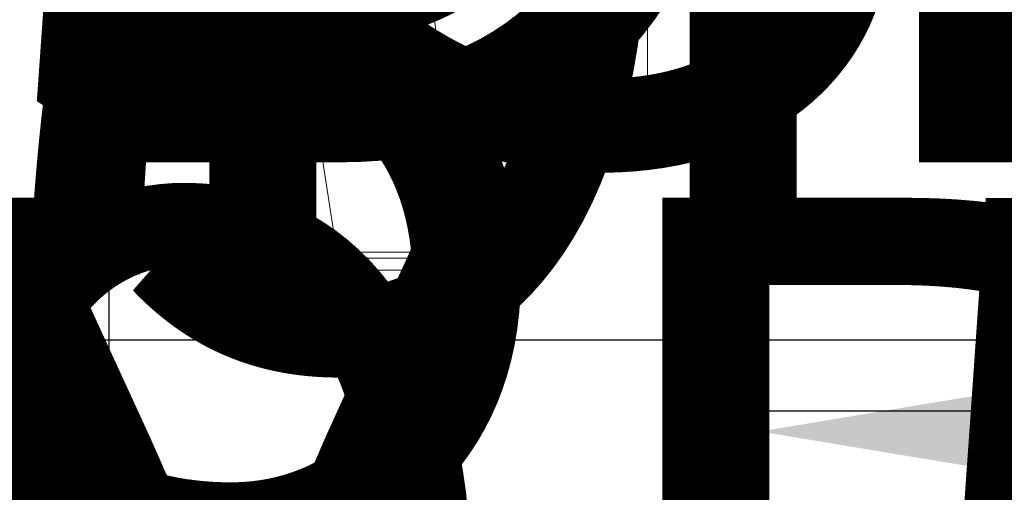
# Model space of a CAD drawing. Units: inches. Extents: x -307 to 2141, y -58 to 895.
# Tile 13 of 28: x 666 to 749, y 396 to 436. Entities that reach past the tile are written whole.
import ezdxf

# ---------------------------------------------------------------- set-up
doc = ezdxf.new("R2010")
doc.units = ezdxf.units.IN
doc.header["$MEASUREMENT"] = 0
doc.layers.add('A-ANNO-DIMS', color=2, linetype='Continuous', lineweight=18)
doc.layers.add('A-FURN', color=8, linetype='Continuous', lineweight=18)
doc.styles.get("Standard").update_dxf_attribs({"font": 'arial.ttf'})
doc.dimstyles.get("Standard").update_dxf_attribs({"dimtxt": 72, "dimasz": 48, "dimexe": 0.18, "dimexo": 0.0625, "dimgap": 0.09, "dimtad": 0, "dimtih": 1, "dimtoh": 1, "dimdec": 0, "dimrnd": 48, "dimzin": 0, "dimdsep": 46, "dimlunit": 3, "dimtxsty": 'Standard', "dimcen": 0.09, "dimadec": 0, "dimazin": 0, "dimtfac": 1, "dimtdec": 0, "dimtofl": 0, "dimtmove": 0, "dimatfit": 3, "dimfxl": 1, "dimtolj": 1, "dimtzin": 0, "dimarcsym": 0})

# ---------------------------------------------------------------- blocks, each defined once
blk = doc.blocks.new('Dining Set - 36 x 72 in.')
for p, q in [((36, 18), (-36, 18)), ((36, -18), (36, 18)), ((44.0006, 8.23428), (35.9976, 9.48474)), ((44, 8.23041), (44, -8.23915)), ((44.5, -8.15843), (44.5, 8.15338)), ((45.5, 8), (44.5005, 8.15617)), ((45.5, 8), (45.5, -8)), ((35.9976, -9.48476), (43.9993, -8.2345)), ((44.4997, -8.15631), (45.5, -8)), ((-36, -18), (36, -18))]:
    blk.add_line(p, q)
for points in [[(22.5879, 15.08984), (24.4721, 14.91715), (26.5052, 14.73958), (28.6809, 14.5581), (30.9929, 14.3737), (33.4347, 14.18733), (36, 14)], [(23.959, 11.37304), (25.2786, 11.08618), (26.8282, 10.76562), (28.6414, 10.40405), (30.752, 9.99414), (33.1936, 9.52856), (36, 9)], [(24.142, 6.64323), (24.4735, 6.70735), (24.8334, 6.75), (25.2235, 6.76969), (25.642, 6.76692), (26.0858, 6.74267), (26.5521, 6.69791), (27.0379, 6.63362), (27.5404, 6.55078), (28.0565, 6.45036), (28.5834, 6.33333), (29.1242, 6.19987), (29.7071, 6.04687), (30.3661, 5.87044), (31.1354, 5.66666), (32.0493, 5.43164), (33.142, 5.16146), (34.4475, 4.85221), (36, 4.5)], [(23.9549, -0.06836), (24.6146, 0.02083), (25.2235, 0.11784), (25.7904, 0.21875), (26.3241, 0.31966), (26.8334, 0.41666), (27.3265, 0.50618), (27.8099, 0.58593), (28.2894, 0.65397), (28.7709, 0.70833), (29.2601, 0.74707), (29.763, 0.76823), (30.2855, 0.76985), (30.8334, 0.75), (31.4088, 0.70784), (31.9994, 0.64713), (32.589, 0.57275), (33.1615, 0.48958), (33.7008, 0.4025), (34.1908, 0.3164), (34.6153, 0.23616), (34.9584, 0.16666), (35.2099, 0.11165), (35.3848, 0.07031), (35.504, 0.04069), (35.5886, 0.02083), (35.6594, 0.00879), (35.7377, 0.0026), (35.8442, 0.00032), (36, 0)], [(23.4727, -4.25391), (24.4289, -4.37549), (25.3334, -4.5), (26.1785, -4.62492), (26.9694, -4.74935), (27.7145, -4.87281), (28.4219, -4.99479), (29.1, -5.11483), (29.7572, -5.23242), (30.4016, -5.34709), (31.0417, -5.45834), (31.6837, -5.56437), (32.3262, -5.65821), (32.9658, -5.73153), (33.599, -5.77604), (34.2224, -5.78345), (34.8327, -5.74545), (35.4264, -5.65373), (36, -5.5)], [(23.9271, -8.76563), (24.9081, -8.82707), (25.8763, -8.89388), (26.8465, -8.96558), (27.8334, -9.04167), (28.8474, -9.12118), (29.8828, -9.20117), (30.93, -9.27824), (31.9792, -9.34896), (33.0205, -9.40991), (34.0443, -9.45768), (35.0407, -9.48885), (36, -9.5)], [(22.6615, -14.44271), (25.2312, -14.21509), (28.2624, -13.9069), (31.8277, -13.50594), (36, -13)]]:
    blk.add_lwpolyline(points)
blk = doc.blocks.new('*D26')
at = {"layer": 'A-ANNO-DIMS', "color": 0, "lineweight": -2, "transparency": 16777216}
for p, q in [((565.336, 584.202), (565.336, 572.085)), ((645.336, 584.202), (645.336, 572.085)), ((517.336, 572.265), (469.336, 572.265)), ((693.336, 572.265), (741.336, 572.265))]:
    blk.add_line(p, q, dxfattribs=at)
at = {"layer": 'A-ANNO-DIMS', "color": 0, "transparency": 16777216}
for points in [[(517.336, 580.265), (517.336, 564.265), (565.336, 572.265)], [(693.336, 580.265), (693.336, 564.265), (645.336, 572.265)]]:
    blk.add_solid(points, dxfattribs=at)
at = {"layer": 'Defpoints', "color": 0, "transparency": 16777216}
for p in [(565.336, 584.265), (645.336, 584.265), (565.336, 572.265)]:
    blk.add_point(p, dxfattribs=at)
at = {"layer": 'A-ANNO-DIMS', "color": 0, "transparency": 16777216, "insert": (178.225, 572.265), "char_height": 72, "attachment_point": 5}
blk.add_mtext('\\A1;BED 80 TYP.', dxfattribs=at)
blk = doc.blocks.new('*D28')
at = {"layer": 'A-ANNO-DIMS', "color": 0, "lineweight": -2, "transparency": 16777216}
for p, q in [((795.358, 433.55), (777.919, 433.55)), ((778.099, 385.55), (778.099, 366.073)), ((795.358, 318.073), (777.919, 318.073)), ((778.099, 318.073), (778.099, 270.073)), ((778.099, 270.073), (730.099, 270.073))]:
    blk.add_line(p, q, dxfattribs=at)
at = {"layer": 'A-ANNO-DIMS', "color": 0, "transparency": 16777216}
for points in [[(770.099, 385.55), (786.099, 385.55), (778.099, 433.55)], [(770.099, 366.073), (786.099, 366.073), (778.099, 318.073)]]:
    blk.add_solid(points, dxfattribs=at)
at = {"layer": 'Defpoints', "color": 0, "transparency": 16777216}
for p in [(795.421, 433.55), (778.099, 318.073), (795.421, 318.073)]:
    blk.add_point(p, dxfattribs=at)
at = {"layer": 'A-ANNO-DIMS', "color": 0, "transparency": 16777216, "insert": (534.416, 270.073), "char_height": 72, "attachment_point": 5}
blk.add_mtext('\\A1;BED 115', dxfattribs=at)
blk = doc.blocks.new('*D29')
at = {"layer": 'A-ANNO-DIMS', "color": 0, "lineweight": -2, "transparency": 16777216}
for p, q in [((747.421, 450.871), (699.421, 450.871)), ((795.421, 433.612), (795.421, 451.051)), ((882.028, 433.612), (882.028, 451.051)), ((930.028, 450.871), (978.028, 450.871))]:
    blk.add_line(p, q, dxfattribs=at)
at = {"layer": 'A-ANNO-DIMS', "color": 0, "transparency": 16777216}
for points in [[(747.421, 458.871), (747.421, 442.871), (795.421, 450.871)], [(930.028, 458.871), (930.028, 442.871), (882.028, 450.871)]]:
    blk.add_solid(points, dxfattribs=at)
at = {"layer": 'Defpoints', "color": 0, "transparency": 16777216}
for p in [(795.421, 450.871), (795.421, 433.55), (882.028, 433.55)]:
    blk.add_point(p, dxfattribs=at)
at = {"layer": 'A-ANNO-DIMS', "color": 0, "transparency": 16777216, "insert": (647.713, 450.871), "char_height": 72, "attachment_point": 5}
blk.add_mtext('\\A1;87', dxfattribs=at)
blk = doc.blocks.new('*D30')
at = {"layer": 'A-ANNO-DIMS', "color": 0, "lineweight": -2, "transparency": 16777216}
for p, q in [((570.736, 532.833), (570.736, 580.833)), ((570.736, 580.833), (618.736, 580.833)), ((565.398, 484.833), (570.916, 484.833)), ((565.398, 448.833), (570.916, 448.833)), ((570.736, 400.833), (570.736, 352.833))]:
    blk.add_line(p, q, dxfattribs=at)
at = {"layer": 'A-ANNO-DIMS', "color": 0, "transparency": 16777216}
for points in [[(562.736, 532.833), (578.736, 532.833), (570.736, 484.833)], [(562.736, 400.833), (578.736, 400.833), (570.736, 448.833)]]:
    blk.add_solid(points, dxfattribs=at)
at = {"layer": 'Defpoints', "color": 0, "transparency": 16777216}
for p in [(565.336, 484.833), (570.736, 484.833), (565.336, 448.833)]:
    blk.add_point(p, dxfattribs=at)
at = {"layer": 'A-ANNO-DIMS', "color": 0, "transparency": 16777216, "insert": (1030.174, 580.833), "char_height": 72, "attachment_point": 5}
blk.add_mtext('\\A1;WINDOW 36 TYP.', dxfattribs=at)
blk = doc.blocks.new('*D31')
at = {"layer": 'A-ANNO-DIMS', "color": 0, "lineweight": -2, "transparency": 16777216}
for p, q in [((556.336, 448.771), (556.336, 443.253)), ((565.336, 448.771), (565.336, 443.253)), ((508.336, 443.433), (460.336, 443.433)), ((613.336, 443.433), (661.336, 443.433))]:
    blk.add_line(p, q, dxfattribs=at)
at = {"layer": 'A-ANNO-DIMS', "color": 0, "transparency": 16777216}
for points in [[(508.336, 451.433), (508.336, 435.433), (556.336, 443.433)], [(613.336, 451.433), (613.336, 435.433), (565.336, 443.433)]]:
    blk.add_solid(points, dxfattribs=at)
at = {"layer": 'Defpoints', "color": 0, "transparency": 16777216}
for p in [(556.336, 448.833), (565.336, 448.833), (565.336, 443.433)]:
    blk.add_point(p, dxfattribs=at)
at = {"layer": 'A-ANNO-DIMS', "color": 0, "transparency": 16777216, "insert": (808.692, 443.433), "char_height": 72, "attachment_point": 5}
blk.add_mtext('\\A1;9 TYP.', dxfattribs=at)
blk = doc.blocks.new('*D35')
at = {"layer": 'A-ANNO-DIMS', "color": 0, "lineweight": -2, "transparency": 16777216}
for p, q in [((907.336, 443.029), (907.336, 453.949)), ((916.336, 443.029), (916.336, 453.949)), ((859.336, 453.769), (811.336, 453.769)), ((964.336, 453.769), (1012.336, 453.769))]:
    blk.add_line(p, q, dxfattribs=at)
at = {"layer": 'A-ANNO-DIMS', "color": 0, "transparency": 16777216}
for points in [[(859.336, 461.769), (859.336, 445.769), (907.336, 453.769)], [(964.336, 461.769), (964.336, 445.769), (916.336, 453.769)]]:
    blk.add_solid(points, dxfattribs=at)
at = {"layer": 'Defpoints', "color": 0, "transparency": 16777216}
for p in [(907.336, 453.769), (907.336, 442.967), (916.336, 442.967)]:
    blk.add_point(p, dxfattribs=at)
at = {"layer": 'A-ANNO-DIMS', "color": 0, "transparency": 16777216, "insert": (663.98, 453.769), "char_height": 72, "attachment_point": 5}
blk.add_mtext('\\A1;9 TYP.', dxfattribs=at)
blk = doc.blocks.new('*D36')
at = {"layer": 'A-ANNO-DIMS', "color": 0, "lineweight": -2, "transparency": 16777216}
for p, q in [((871.707, 562.404), (871.761, 610.404)), ((876.548, 514.399), (871.474, 514.405)), ((876.511, 481.353), (871.437, 481.358)), ((871.563, 433.358), (871.509, 385.358)), ((871.509, 385.358), (823.509, 385.358))]:
    blk.add_line(p, q, dxfattribs=at)
at = {"layer": 'A-ANNO-DIMS', "color": 0, "transparency": 16777216}
for points in [[(863.707, 562.413), (879.707, 562.395), (871.654, 514.404)], [(863.563, 433.367), (879.563, 433.349), (871.617, 481.358)]]:
    blk.add_solid(points, dxfattribs=at)
at = {"layer": 'Defpoints', "color": 0, "transparency": 16777216}
for p in [(876.611, 514.399), (871.617, 481.358), (876.574, 481.353)]:
    blk.add_point(p, dxfattribs=at)
at = {"layer": 'A-ANNO-DIMS', "color": 0, "transparency": 16777216, "insert": (548.95, 385.358), "char_height": 72, "attachment_point": 5}
blk.add_mtext('\\A1;WC 33 TYP.', dxfattribs=at)
blk = doc.blocks.new('*D37')
at = {"layer": 'A-ANNO-DIMS', "color": 0, "lineweight": -2, "transparency": 16777216}
for p, q in [((828.616, 519.409), (780.616, 519.463)), ((876.611, 514.461), (876.616, 519.536)), ((897.611, 514.438), (897.616, 519.512)), ((945.616, 519.279), (993.616, 519.225))]:
    blk.add_line(p, q, dxfattribs=at)
at = {"layer": 'A-ANNO-DIMS', "color": 0, "transparency": 16777216}
for points in [[(828.625, 527.409), (828.607, 511.409), (876.616, 519.356)], [(945.625, 527.279), (945.607, 511.279), (897.616, 519.332)]]:
    blk.add_solid(points, dxfattribs=at)
at = {"layer": 'Defpoints', "color": 0, "transparency": 16777216}
for p in [(876.616, 519.356), (876.611, 514.399), (897.611, 514.375)]:
    blk.add_point(p, dxfattribs=at)
at = {"layer": 'A-ANNO-DIMS', "color": 0, "transparency": 16777216, "insert": (604.676, 519.463), "char_height": 72, "attachment_point": 5}
blk.add_mtext('\\A1;21 TYP.', dxfattribs=at)
blk = doc.blocks.new('*D44')
at = {"layer": 'A-ANNO-DIMS', "color": 0, "lineweight": -2, "transparency": 16777216}
for p, q in [((815.327, 520.707), (815.406, 516.907)), ((839.872, 521.223), (839.952, 517.424)), ((887.938, 518.613), (935.927, 519.622)), ((767.413, 516.078), (719.424, 515.069))]:
    blk.add_line(p, q, dxfattribs=at)
at = {"layer": 'A-ANNO-DIMS', "color": 0, "transparency": 16777216}
for points in [[(887.769, 526.611), (888.106, 510.614), (839.948, 517.604)], [(767.245, 524.076), (767.581, 508.08), (815.403, 517.087)]]:
    blk.add_solid(points, dxfattribs=at)
at = {"layer": 'Defpoints', "color": 0, "transparency": 16777216}
for p in [(815.325, 520.769), (839.871, 521.285), (839.948, 517.604)]:
    blk.add_point(p, dxfattribs=at)
at = {"layer": 'A-ANNO-DIMS', "color": 0, "transparency": 16777216, "insert": (1151.157, 519.622), "char_height": 72, "attachment_point": 5}
blk.add_mtext('\\A1;BASIN 25', dxfattribs=at)
blk = doc.blocks.new('*D45')
at = {"layer": 'A-ANNO-DIMS', "color": 0, "lineweight": -2, "transparency": 16777216}
for p, q in [((841.111, 637.474), (793.111, 637.474)), ((842.12, 589.484), (841.111, 637.474)), ((839.51, 541.419), (843.309, 541.499)), ((839.933, 521.287), (843.732, 521.367)), ((844.562, 473.373), (845.571, 425.384))]:
    blk.add_line(p, q, dxfattribs=at)
at = {"layer": 'A-ANNO-DIMS', "color": 0, "transparency": 16777216}
for points in [[(850.118, 589.652), (834.122, 589.316), (843.129, 541.495)], [(852.56, 473.542), (836.563, 473.205), (843.553, 521.363)]]:
    blk.add_solid(points, dxfattribs=at)
at = {"layer": 'Defpoints', "color": 0, "transparency": 16777216}
for p in [(839.447, 541.417), (843.129, 541.495), (839.871, 521.285)]:
    blk.add_point(p, dxfattribs=at)
at = {"layer": 'A-ANNO-DIMS', "color": 0, "transparency": 16777216, "insert": (740.961, 637.474), "char_height": 72, "attachment_point": 5}
blk.add_mtext('\\A1;20', dxfattribs=at)
blk = doc.blocks.new('*D50')
at = {"layer": 'A-ANNO-DIMS', "color": 0, "lineweight": -2, "transparency": 16777216}
for p, q in [((565.336, 315.804), (565.336, 313.146)), ((582.271, 315.804), (582.271, 313.146)), ((517.336, 313.326), (469.336, 313.326)), ((630.271, 313.326), (678.271, 313.326))]:
    blk.add_line(p, q, dxfattribs=at)
at = {"layer": 'A-ANNO-DIMS', "color": 0, "transparency": 16777216}
for points in [[(517.336, 321.326), (517.336, 305.326), (565.336, 313.326)], [(630.271, 321.326), (630.271, 305.326), (582.271, 313.326)]]:
    blk.add_solid(points, dxfattribs=at)
at = {"layer": 'Defpoints', "color": 0, "transparency": 16777216}
for p in [(565.336, 315.867), (582.271, 315.867), (565.336, 313.326)]:
    blk.add_point(p, dxfattribs=at)
at = {"layer": 'A-ANNO-DIMS', "color": 0, "transparency": 16777216, "insert": (226.651, 313.326), "char_height": 72, "attachment_point": 5}
blk.add_mtext('\\A1;PHONE 17', dxfattribs=at)
blk = doc.blocks.new('*D51')
at = {"layer": 'A-ANNO-DIMS', "color": 0, "lineweight": -2, "transparency": 16777216}
for p, q in [((562.796, 379.109), (562.796, 427.109)), ((562.796, 427.109), (610.796, 427.109)), ((565.273, 331.109), (562.616, 331.109)), ((565.273, 315.867), (562.616, 315.867)), ((562.796, 267.867), (562.796, 219.867))]:
    blk.add_line(p, q, dxfattribs=at)
at = {"layer": 'A-ANNO-DIMS', "color": 0, "transparency": 16777216}
for points in [[(554.796, 379.109), (570.796, 379.109), (562.796, 331.109)], [(554.796, 267.867), (570.796, 267.867), (562.796, 315.867)]]:
    blk.add_solid(points, dxfattribs=at)
at = {"layer": 'Defpoints', "color": 0, "transparency": 16777216}
for p in [(562.796, 331.109), (565.336, 331.109), (565.336, 315.867)]:
    blk.add_point(p, dxfattribs=at)
at = {"layer": 'A-ANNO-DIMS', "color": 0, "transparency": 16777216, "insert": (659.336, 427.109), "char_height": 72, "attachment_point": 5}
blk.add_mtext('\\A1;15', dxfattribs=at)
blk = doc.blocks.new('*D52')
at = {"layer": 'A-ANNO-DIMS', "color": 0, "lineweight": -2, "transparency": 16777216}
for p, q in [((660.208, 554.249), (660.208, 602.249)), ((673.796, 506.249), (660.028, 506.249)), ((673.796, 415.249), (660.028, 415.249)), ((660.208, 367.249), (660.208, 319.249))]:
    blk.add_line(p, q, dxfattribs=at)
at = {"layer": 'A-ANNO-DIMS', "color": 0, "transparency": 16777216}
for points in [[(652.208, 554.249), (668.208, 554.249), (660.208, 506.249)], [(652.208, 367.249), (668.208, 367.249), (660.208, 415.249)]]:
    blk.add_solid(points, dxfattribs=at)
at = {"layer": 'Defpoints', "color": 0, "transparency": 16777216}
for p in [(673.858, 506.249), (660.208, 415.249), (673.858, 415.249)]:
    blk.add_point(p, dxfattribs=at)
at = {"layer": 'A-ANNO-DIMS', "color": 0, "transparency": 16777216, "insert": (660.208, 460.749), "char_height": 72, "attachment_point": 5}
blk.add_mtext('\\A1;DINING SET 91', dxfattribs=at)
blk = doc.blocks.new('*D53')
at = {"layer": 'A-ANNO-DIMS', "color": 0, "lineweight": -2, "transparency": 16777216}
for p, q in [((673.858, 415.186), (673.858, 401.419)), ((728.858, 415.186), (728.858, 401.419)), ((625.858, 401.599), (577.858, 401.599)), ((776.858, 401.599), (824.858, 401.599))]:
    blk.add_line(p, q, dxfattribs=at)
at = {"layer": 'A-ANNO-DIMS', "color": 0, "transparency": 16777216}
for points in [[(625.858, 409.599), (625.858, 393.599), (673.858, 401.599)], [(776.858, 409.599), (776.858, 393.599), (728.858, 401.599)]]:
    blk.add_solid(points, dxfattribs=at)
at = {"layer": 'Defpoints', "color": 0, "transparency": 16777216}
for p in [(673.858, 415.249), (728.858, 415.249), (728.858, 401.599)]:
    blk.add_point(p, dxfattribs=at)
at = {"layer": 'A-ANNO-DIMS', "color": 0, "transparency": 16777216, "insert": (876.787, 401.599), "char_height": 72, "attachment_point": 5}
blk.add_mtext('\\A1;55', dxfattribs=at)
blk = doc.blocks.new('*D54')
at = {"layer": 'A-ANNO-DIMS', "color": 0, "lineweight": -2, "transparency": 16777216}
for p, q in [((605.336, 412.349), (605.336, 460.349)), ((605.336, 460.349), (653.336, 460.349)), ((596.398, 364.349), (605.516, 364.349)), ((596.398, 304.349), (605.516, 304.349)), ((605.336, 256.349), (605.336, 208.349))]:
    blk.add_line(p, q, dxfattribs=at)
at = {"layer": 'A-ANNO-DIMS', "color": 0, "transparency": 16777216}
for points in [[(597.336, 412.349), (613.336, 412.349), (605.336, 364.349)], [(597.336, 256.349), (613.336, 256.349), (605.336, 304.349)]]:
    blk.add_solid(points, dxfattribs=at)
at = {"layer": 'Defpoints', "color": 0, "transparency": 16777216}
for p in [(596.336, 364.349), (605.336, 364.349), (596.336, 304.349)]:
    blk.add_point(p, dxfattribs=at)
at = {"layer": 'A-ANNO-DIMS', "color": 0, "transparency": 16777216, "insert": (854.004, 460.349), "char_height": 72, "attachment_point": 5}
blk.add_mtext('\\A1;DESK 60', dxfattribs=at)
blk = doc.blocks.new('*D55')
at = {"layer": 'A-ANNO-DIMS', "color": 0, "lineweight": -2, "transparency": 16777216}
for p, q in [((517.336, 373.349), (469.336, 373.349)), ((565.336, 364.411), (565.336, 373.529)), ((596.336, 364.411), (596.336, 373.529)), ((644.336, 373.349), (692.336, 373.349))]:
    blk.add_line(p, q, dxfattribs=at)
at = {"layer": 'A-ANNO-DIMS', "color": 0, "transparency": 16777216}
for points in [[(517.336, 381.349), (517.336, 365.349), (565.336, 373.349)], [(644.336, 381.349), (644.336, 365.349), (596.336, 373.349)]]:
    blk.add_solid(points, dxfattribs=at)
at = {"layer": 'Defpoints', "color": 0, "transparency": 16777216}
for p in [(565.336, 373.349), (565.336, 364.349), (596.336, 364.349)]:
    blk.add_point(p, dxfattribs=at)
at = {"layer": 'A-ANNO-DIMS', "color": 0, "transparency": 16777216, "insert": (424.651, 373.349), "char_height": 72, "attachment_point": 5}
blk.add_mtext('\\A1;31', dxfattribs=at)
blk = doc.blocks.new('*D60')
at = {"layer": 'A-ANNO-DIMS', "color": 0, "lineweight": -2, "transparency": 16777216}
for p, q in [((659.857, 294.946), (659.857, 342.946)), ((659.857, 342.946), (707.857, 342.946)), ((663.339, 246.946), (659.677, 246.946)), ((663.339, 223.315), (659.677, 223.315)), ((659.857, 175.315), (659.857, 127.315))]:
    blk.add_line(p, q, dxfattribs=at)
at = {"layer": 'A-ANNO-DIMS', "color": 0, "transparency": 16777216}
for points in [[(651.857, 294.946), (667.857, 294.946), (659.857, 246.946)], [(651.857, 175.315), (667.857, 175.315), (659.857, 223.315)]]:
    blk.add_solid(points, dxfattribs=at)
at = {"layer": 'Defpoints', "color": 0, "transparency": 16777216}
for p in [(659.857, 246.946), (663.402, 246.946), (663.402, 223.315)]:
    blk.add_point(p, dxfattribs=at)
at = {"layer": 'A-ANNO-DIMS', "color": 0, "transparency": 16777216, "insert": (933.573, 342.946), "char_height": 72, "attachment_point": 5}
blk.add_mtext('\\A1;TABLE 24', dxfattribs=at)
blk = doc.blocks.new('*D63')
at = {"layer": 'A-ANNO-DIMS', "color": 0, "lineweight": -2, "transparency": 16777216}
for p, q in [((916.398, 691.341), (947.72, 691.341)), ((947.54, 643.341), (947.54, 416.192)), ((947.54, 115.341), (947.54, 342.49)), ((704.684, 67.341), (947.72, 67.341))]:
    blk.add_line(p, q, dxfattribs=at)
at = {"layer": 'A-ANNO-DIMS', "color": 0, "transparency": 16777216}
for points in [[(939.54, 643.341), (955.54, 643.341), (947.54, 691.341)], [(939.54, 115.341), (955.54, 115.341), (947.54, 67.341)]]:
    blk.add_solid(points, dxfattribs=at)
at = {"layer": 'Defpoints', "color": 0, "transparency": 16777216}
for p in [(916.336, 691.341), (704.621, 67.341), (947.54, 67.341)]:
    blk.add_point(p, dxfattribs=at)
at = {"layer": 'A-ANNO-DIMS', "color": 0, "transparency": 16777216, "insert": (947.54, 379.341), "char_height": 72, "attachment_point": 5}
blk.add_mtext('\\A1;624', dxfattribs=at)
blk = doc.blocks.new('*D68')
at = {"layer": 'A-ANNO-DIMS', "color": 0, "lineweight": -2, "transparency": 16777216}
for p, q in [((525.132, 586.341), (525.132, 634.341)), ((525.132, 634.341), (573.132, 634.341)), ((565.273, 538.341), (524.952, 538.341)), ((556.273, 484.833), (524.952, 484.833)), ((525.132, 436.833), (525.132, 388.833))]:
    blk.add_line(p, q, dxfattribs=at)
at = {"layer": 'A-ANNO-DIMS', "color": 0, "transparency": 16777216}
for points in [[(517.132, 586.341), (533.132, 586.341), (525.132, 538.341)], [(517.132, 436.833), (533.132, 436.833), (525.132, 484.833)]]:
    blk.add_solid(points, dxfattribs=at)
at = {"layer": 'Defpoints', "color": 0, "transparency": 16777216}
for p in [(525.132, 538.341), (565.336, 538.341), (556.336, 484.833)]:
    blk.add_point(p, dxfattribs=at)
at = {"layer": 'A-ANNO-DIMS', "color": 0, "transparency": 16777216, "insert": (687.754, 634.341), "char_height": 72, "attachment_point": 5}
blk.add_mtext('\\A1;53.51', dxfattribs=at)
blk = doc.blocks.new('*D82')
at = {"layer": 'A-ANNO-DIMS', "color": 0, "lineweight": -2, "transparency": 16777216}
for p, q in [((525.132, 565.341), (525.132, 613.341)), ((525.132, 613.341), (573.132, 613.341)), ((802.273, 517.341), (524.952, 517.341)), ((802.273, 481.341), (524.952, 481.341)), ((525.132, 433.341), (525.132, 385.341))]:
    blk.add_line(p, q, dxfattribs=at)
at = {"layer": 'A-ANNO-DIMS', "color": 0, "transparency": 16777216}
for points in [[(517.132, 565.341), (533.132, 565.341), (525.132, 517.341)], [(517.132, 433.341), (533.132, 433.341), (525.132, 481.341)]]:
    blk.add_solid(points, dxfattribs=at)
at = {"layer": 'Defpoints', "color": 0, "transparency": 16777216}
for p in [(525.132, 517.341), (802.336, 517.341), (802.336, 481.341)]:
    blk.add_point(p, dxfattribs=at)
at = {"layer": 'A-ANNO-DIMS', "color": 0, "transparency": 16777216, "insert": (624.742, 613.341), "char_height": 72, "attachment_point": 5}
blk.add_mtext('\\A1;36', dxfattribs=at)
blk = doc.blocks.new('*D83')
at = {"layer": 'A-ANNO-DIMS', "color": 0, "lineweight": -2, "transparency": 16777216}
for p, q in [((947.54, 538.903), (947.54, 586.903)), ((916.398, 490.903), (947.72, 490.903)), ((907.398, 481.341), (947.72, 481.341)), ((947.54, 433.341), (947.54, 385.341)), ((947.54, 385.341), (899.54, 385.341))]:
    blk.add_line(p, q, dxfattribs=at)
at = {"layer": 'A-ANNO-DIMS', "color": 0, "transparency": 16777216}
for points in [[(939.54, 538.903), (955.54, 538.903), (947.54, 490.903)], [(939.54, 433.341), (955.54, 433.341), (947.54, 481.341)]]:
    blk.add_solid(points, dxfattribs=at)
at = {"layer": 'Defpoints', "color": 0, "transparency": 16777216}
for p in [(916.336, 490.903), (907.336, 481.341), (947.54, 481.341)]:
    blk.add_point(p, dxfattribs=at)
at = {"layer": 'A-ANNO-DIMS', "color": 0, "transparency": 16777216, "insert": (777.968, 385.341), "char_height": 72, "attachment_point": 5}
blk.add_mtext('\\A1;9.563', dxfattribs=at)
blk = doc.blocks.new('*D88')
at = {"layer": 'A-ANNO-DIMS', "color": 0, "lineweight": -2, "transparency": 16777216}
for p, q in [((517.33584, 722.544828), (469.33584, 722.544828)), ((565.33584, 295.403328), (565.33584, 722.724828)), ((754.33584, 271.403328), (754.33584, 722.724828)), ((802.33584, 722.544828), (850.33584, 722.544828))]:
    blk.add_line(p, q, dxfattribs=at)
at = {"layer": 'A-ANNO-DIMS', "color": 0, "transparency": 16777216}
for points in [[(517.33584, 730.544828), (517.33584, 714.544828), (565.33584, 722.544828)], [(802.33584, 730.544828), (802.33584, 714.544828), (754.33584, 722.544828)]]:
    blk.add_solid(points, dxfattribs=at)
at = {"layer": 'Defpoints', "color": 0, "transparency": 16777216}
for p in [(754.33584, 722.544828), (565.33584, 295.340828), (754.33584, 271.340828)]:
    blk.add_point(p, dxfattribs=at)
at = {"layer": 'A-ANNO-DIMS', "color": 0, "transparency": 16777216, "insert": (659.83584, 722.544828), "char_height": 72, "attachment_point": 5}
blk.add_mtext('\\A1;189', dxfattribs=at)
blk = doc.blocks.new('*D95')
at = {"layer": 'A-ANNO-DIMS', "color": 0, "lineweight": -2, "transparency": 16777216}
for p, q in [((947.54, 577.341), (947.54, 625.341)), ((947.54, 625.341), (995.54, 625.341)), ((629.898, 529.341), (947.72, 529.341)), ((629.898, 502.663), (947.72, 502.663)), ((947.54, 454.663), (947.54, 406.663))]:
    blk.add_line(p, q, dxfattribs=at)
at = {"layer": 'A-ANNO-DIMS', "color": 0, "transparency": 16777216}
for points in [[(939.54, 577.341), (955.54, 577.341), (947.54, 529.341)], [(939.54, 454.663), (955.54, 454.663), (947.54, 502.663)]]:
    blk.add_solid(points, dxfattribs=at)
at = {"layer": 'Defpoints', "color": 0, "transparency": 16777216}
for p in [(629.836, 529.341), (947.54, 529.341), (629.836, 502.663)]:
    blk.add_point(p, dxfattribs=at)
at = {"layer": 'A-ANNO-DIMS', "color": 0, "transparency": 16777216, "insert": (1117.799, 625.341), "char_height": 72, "attachment_point": 5}
blk.add_mtext('\\A1;26.68', dxfattribs=at)
blk = doc.blocks.new('*D99')
at = {"layer": 'A-ANNO-DIMS', "color": 0, "lineweight": -2, "transparency": 16777216}
for p, q in [((763.336, 481.278), (763.336, 35.957)), ((802.336, 481.278), (802.336, 35.957)), ((715.336, 36.137), (667.336, 36.137)), ((850.336, 36.137), (898.336, 36.137))]:
    blk.add_line(p, q, dxfattribs=at)
at = {"layer": 'A-ANNO-DIMS', "color": 0, "transparency": 16777216}
for points in [[(715.336, 44.137), (715.336, 28.137), (763.336, 36.137)], [(850.336, 44.137), (850.336, 28.137), (802.336, 36.137)]]:
    blk.add_solid(points, dxfattribs=at)
at = {"layer": 'Defpoints', "color": 0, "transparency": 16777216}
for p in [(763.336, 481.341), (802.336, 481.341), (802.336, 36.137)]:
    blk.add_point(p, dxfattribs=at)
at = {"layer": 'A-ANNO-DIMS', "color": 0, "transparency": 16777216, "insert": (950.044, 36.137), "char_height": 72, "attachment_point": 5}
blk.add_mtext('\\A1;39', dxfattribs=at)
blk = doc.blocks.new('*D100')
at = {"layer": 'A-ANNO-DIMS', "color": 0, "lineweight": -2, "transparency": 16777216}
for p, q in [((589.339, 409.278), (589.339, 35.957)), ((625.336, 409.278), (625.336, 35.957)), ((541.339, 36.137), (493.339, 36.137)), ((673.336, 36.137), (721.336, 36.137))]:
    blk.add_line(p, q, dxfattribs=at)
at = {"layer": 'A-ANNO-DIMS', "color": 0, "transparency": 16777216}
for points in [[(541.339, 44.137), (541.339, 28.137), (589.339, 36.137)], [(673.336, 44.137), (673.336, 28.137), (625.336, 36.137)]]:
    blk.add_solid(points, dxfattribs=at)
at = {"layer": 'Defpoints', "color": 0, "transparency": 16777216}
for p in [(589.339, 409.341), (625.336, 409.341), (625.336, 36.137)]:
    blk.add_point(p, dxfattribs=at)
at = {"layer": 'A-ANNO-DIMS', "color": 0, "transparency": 16777216, "insert": (772.946, 36.137), "char_height": 72, "attachment_point": 5}
blk.add_mtext('\\A1;36', dxfattribs=at)
blk = doc.blocks.new('*D107')
at = {"layer": 'A-ANNO-DIMS', "color": 0, "lineweight": -2, "transparency": 16777216}
for p, q in [((517.336, 722.545), (469.336, 722.545)), ((565.336, 409.403), (565.336, 722.725)), ((589.339, 409.403), (589.339, 722.725)), ((637.339, 722.545), (685.339, 722.545))]:
    blk.add_line(p, q, dxfattribs=at)
at = {"layer": 'A-ANNO-DIMS', "color": 0, "transparency": 16777216}
for points in [[(517.336, 730.545), (517.336, 714.545), (565.336, 722.545)], [(637.339, 730.545), (637.339, 714.545), (589.339, 722.545)]]:
    blk.add_solid(points, dxfattribs=at)
at = {"layer": 'Defpoints', "color": 0, "transparency": 16777216}
for p in [(589.339, 722.545), (565.336, 409.341), (589.339, 409.341)]:
    blk.add_point(p, dxfattribs=at)
at = {"layer": 'A-ANNO-DIMS', "color": 0, "transparency": 16777216, "insert": (835.495, 722.545), "char_height": 72, "attachment_point": 5}
blk.add_mtext('\\A1;24.003', dxfattribs=at)
blk = doc.blocks.new('*D108')
at = {"layer": 'A-ANNO-DIMS', "color": 0, "lineweight": -2, "transparency": 16777216}
for p, q in [((947.54, 550.663), (947.54, 598.663)), ((589.402, 502.663), (947.72, 502.663)), ((589.402, 409.341), (947.72, 409.341)), ((947.54, 361.341), (947.54, 313.341))]:
    blk.add_line(p, q, dxfattribs=at)
at = {"layer": 'A-ANNO-DIMS', "color": 0, "transparency": 16777216}
for points in [[(939.54, 550.663), (955.54, 550.663), (947.54, 502.663)], [(939.54, 361.341), (955.54, 361.341), (947.54, 409.341)]]:
    blk.add_solid(points, dxfattribs=at)
at = {"layer": 'Defpoints', "color": 0, "transparency": 16777216}
for p in [(589.339, 502.663), (947.54, 502.663), (589.339, 409.341)]:
    blk.add_point(p, dxfattribs=at)
at = {"layer": 'A-ANNO-DIMS', "color": 0, "transparency": 16777216, "insert": (947.54, 456.002), "char_height": 72, "attachment_point": 5}
blk.add_mtext('\\A1;93.32', dxfattribs=at)
blk = doc.blocks.new('*D109')
at = {"layer": 'A-ANNO-DIMS', "color": 0, "lineweight": -2, "transparency": 16777216}
for p, q in [((723.132, 355.341), (723.132, 403.341)), ((723.132, 403.341), (771.132, 403.341)), ((754.273, 307.341), (722.952, 307.341)), ((754.273, 271.341), (722.952, 271.341)), ((723.132, 223.341), (723.132, 175.341))]:
    blk.add_line(p, q, dxfattribs=at)
at = {"layer": 'A-ANNO-DIMS', "color": 0, "transparency": 16777216}
for points in [[(715.132, 355.341), (731.132, 355.341), (723.132, 307.341)], [(715.132, 223.341), (731.132, 223.341), (723.132, 271.341)]]:
    blk.add_solid(points, dxfattribs=at)
at = {"layer": 'Defpoints', "color": 0, "transparency": 16777216}
for p in [(723.132, 307.341), (754.336, 307.341), (754.336, 271.341)]:
    blk.add_point(p, dxfattribs=at)
at = {"layer": 'A-ANNO-DIMS', "color": 0, "transparency": 16777216, "insert": (822.742, 403.341), "char_height": 72, "attachment_point": 5}
blk.add_mtext('\\A1;36', dxfattribs=at)

msp = doc.modelspace()

# ---------------------------------------------------------------- block references
at = {"layer": 'A-FURN', "rotation": 270}
msp.add_blockref('Dining Set - 36 x 72 in.', (701.3583, 460.7485), dxfattribs=at)

# ---------------------------------------------------------------- dimensions: what is measured, and where the dimension line sits
at = {"layer": 'A-ANNO-DIMS'}
for base, p1, p2, override, picture, middle in [((754.3358, 722.5448), (565.3358, 295.3408), (754.3358, 271.3408), {"dimdec": 0, "dimlfac": 1, "dimrnd": 0, "dimzin": 0, "dimdsep": 46, "dimlunit": 2}, '*D88', (659.8358, 722.5448)), ((589.339, 722.5448), (565.3358, 409.3408), (589.339, 409.3408), {"dimdec": 3, "dimlfac": 1, "dimrnd": 0, "dimzin": 0, "dimdsep": 46, "dimlunit": 2}, '*D107', (835.4945, 722.5448)), ((802.3358, 36.1368), (763.3358, 481.3408), (802.3358, 481.3408), {"dimdec": 0, "dimlfac": 1, "dimrnd": 0, "dimzin": 0, "dimdsep": 46, "dimlunit": 2}, '*D99', (950.0438, 36.1368)), ((728.8583, 401.5985), (673.8583, 415.2485), (728.8583, 415.2485), {"dimdec": 0, "dimlfac": 1, "dimrnd": 0, "dimzin": 0, "dimdsep": 46, "dimlunit": 2}, '*D53', (876.7874, 401.5985)), ((625.3358, 36.1368), (589.339, 409.3408), (625.3358, 409.3408), {"dimdec": 0, "dimlfac": 1, "dimrnd": 0, "dimzin": 0, "dimdsep": 46, "dimlunit": 2}, '*D100', (772.9456, 36.1368))]:
    dim = msp.add_linear_dim(base=base, p1=p1, p2=p2, dimstyle='Standard', override=override, dxfattribs=at)
    dim.commit()
    dim.dimension.update_dxf_attribs({"geometry": picture, "text_midpoint": middle})
for base, p1, p2, angle, text, picture, middle in [((570.7358, 484.8333), (565.3358, 448.8333), (565.3358, 484.8333), 90, 'WINDOW <> TYP.', '*D30', (1030.1737, 580.8333)), ((565.3358, 572.2648), (645.3359, 584.2648), (565.3358, 584.2648), 180, 'BED <> TYP.', '*D26', (178.2254, 572.2648)), ((660.2083, 415.2485), (673.8583, 506.2485), (673.8583, 415.2485), 270, 'DINING SET <>', '*D52', (660.2083, 460.7485)), ((839.9481, 517.6035), (815.3253, 520.7692), (839.8707, 521.2853), 1.204628, 'BASIN <>', '*D44', (1151.1574, 519.6217)), ((876.6162, 519.3557), (897.6106, 514.3753), (876.6106, 514.3988), 179.935892, '<> TYP.', '*D37', (604.6763, 519.4631)), ((871.6167, 481.3581), (876.6106, 514.3988), (876.5736, 481.3526), 269.935892, 'WC <> TYP.', '*D36', (548.95, 385.3582)), ((605.3358, 364.3488), (596.3358, 304.3488), (596.3358, 364.3488), 90, 'DESK <>', '*D54', (854.0043, 460.3488)), ((907.3358, 453.7692), (916.3358, 442.9669), (907.3358, 442.9669), 180, '<> TYP.', '*D35', (663.9798, 453.7692)), ((659.8571, 246.9465), (663.4018, 223.3153), (663.4018, 246.9465), 90, 'TABLE <>', '*D60', (933.5733, 342.9465)), ((778.0993, 318.073), (795.4208, 433.5496), (795.4208, 318.073), 270, 'BED <>', '*D28', (534.4158, 270.073)), ((565.3358, 313.3263), (582.2714, 315.8666), (565.3358, 315.8666), 180, 'PHONE <>', '*D50', (226.651, 313.3263))]:
    dim = msp.add_linear_dim(base=base, p1=p1, p2=p2, angle=angle, text=text, dimstyle='Standard', override={"dimdec": 0, "dimlfac": 1, "dimrnd": 0, "dimzin": 0, "dimdsep": 46, "dimlunit": 2}, dxfattribs=at)
    dim.commit()
    dim.dimension.update_dxf_attribs({"geometry": picture, "text_midpoint": middle})
for base, p1, p2, angle, override, picture, middle in [((947.5398, 67.3408), (916.3358, 691.3408), (704.6211, 67.3408), 90, {"dimdec": 0, "dimlfac": 1, "dimrnd": 0, "dimzin": 0, "dimdsep": 46, "dimlunit": 2}, '*D63', (947.5398, 379.3408)), ((843.1292, 541.4949), (839.8707, 521.2853), (839.4474, 541.4175), 91.204628, {"dimdec": 0, "dimlfac": 1, "dimrnd": 0, "dimzin": 0, "dimdsep": 46, "dimlunit": 2}, '*D45', (740.961, 637.4737)), ((525.1318, 538.3408), (556.3358, 484.8333), (565.3358, 538.3408), 90, {"dimdec": 2, "dimlfac": 1, "dimrnd": 0, "dimzin": 0, "dimdsep": 46, "dimlunit": 2}, '*D68', (687.7539, 634.3408)), ((947.5398, 529.3408), (629.8358, 502.6632), (629.8358, 529.3408), 90, {"dimdec": 2, "dimlfac": 1, "dimrnd": 0, "dimzin": 0, "dimdsep": 46, "dimlunit": 2}, '*D95', (1117.799, 625.3408)), ((525.1318, 517.3408), (802.3358, 481.3408), (802.3358, 517.3408), 90, {"dimdec": 0, "dimlfac": 1, "dimrnd": 0, "dimzin": 0, "dimdsep": 46, "dimlunit": 2}, '*D82', (624.7416, 613.3408)), ((947.5398, 502.6632), (589.339, 409.3408), (589.339, 502.6632), 90, {"dimdec": 2, "dimlfac": 1, "dimrnd": 0, "dimzin": 0, "dimdsep": 46, "dimlunit": 2}, '*D108', (947.5398, 456.002)), ((947.5398, 481.3408), (916.3358, 490.9034), (907.3358, 481.3408), 90, {"dimdec": 3, "dimlfac": 1, "dimrnd": 0, "dimzin": 0, "dimdsep": 46, "dimlunit": 2}, '*D83', (777.9683, 385.3408)), ((795.4208, 450.8711), (882.0282, 433.5496), (795.4208, 433.5496), 180, {"dimdec": 0, "dimlfac": 1, "dimrnd": 0, "dimzin": 0, "dimdsep": 46, "dimlunit": 2}, '*D29', (647.7128, 450.8711)), ((562.7955, 331.1086), (565.3358, 315.8666), (565.3358, 331.1086), 90, {"dimdec": 0, "dimlfac": 1, "dimrnd": 0, "dimzin": 0, "dimdsep": 46, "dimlunit": 2}, '*D51', (659.3357, 427.1086)), ((723.1318, 307.3408), (754.3358, 271.3408), (754.3358, 307.3408), 90, {"dimdec": 0, "dimlfac": 1, "dimrnd": 0, "dimzin": 0, "dimdsep": 46, "dimlunit": 2}, '*D109', (822.7416, 403.3408)), ((565.3358, 373.3488), (596.3358, 364.3488), (565.3358, 364.3488), 180, {"dimdec": 0, "dimlfac": 1, "dimrnd": 0, "dimzin": 0, "dimdsep": 46, "dimlunit": 2}, '*D55', (424.651, 373.3488))]:
    dim = msp.add_linear_dim(base=base, p1=p1, p2=p2, angle=angle, dimstyle='Standard', override=override, dxfattribs=at)
    dim.commit()
    dim.dimension.update_dxf_attribs({"geometry": picture, "text_midpoint": middle})
dim = msp.add_linear_dim(base=(565.3358, 443.4333), p1=(556.3358, 448.8333), p2=(565.3358, 448.8333), text='<> TYP.', dimstyle='Standard', override={"dimdec": 0, "dimlfac": 1, "dimrnd": 0, "dimzin": 0, "dimdsep": 46, "dimlunit": 2}, dxfattribs=at)
dim.commit()
dim.dimension.update_dxf_attribs({"geometry": '*D31', "text_midpoint": (808.6919, 443.4333)})

doc.saveas('drawing.dxf')
